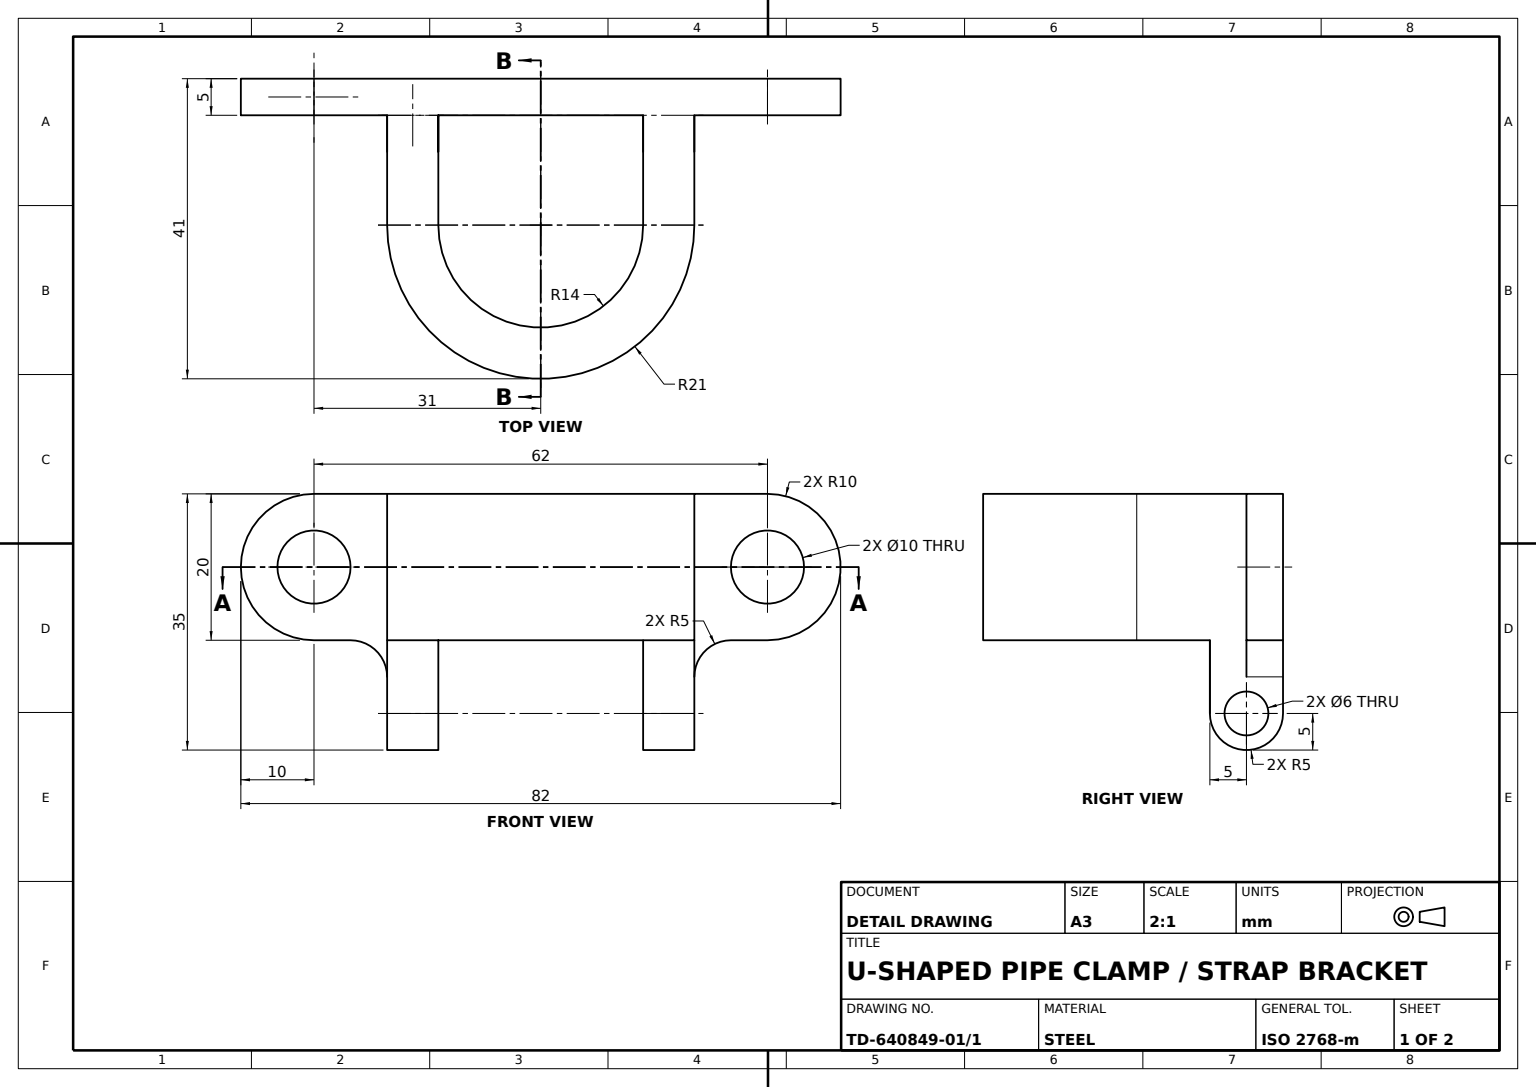
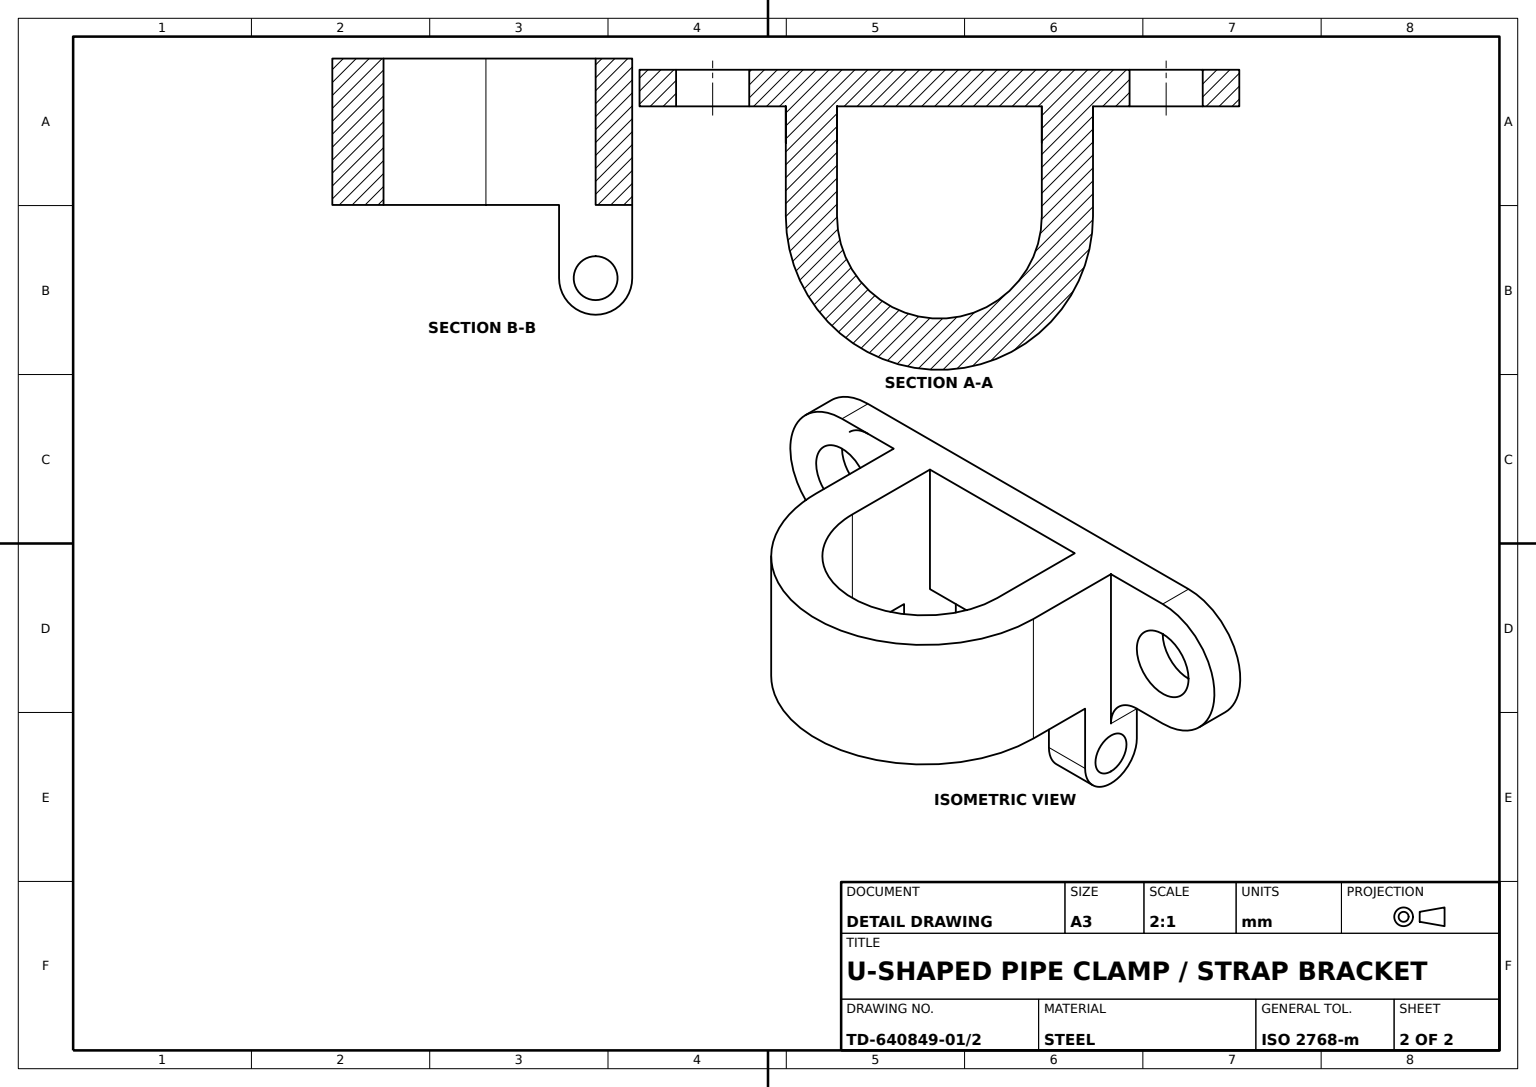
from build123d import *

# Parameters (mm, degrees)
BASE_FLANGE_DEPTH        = 5
CLAMP_BODY_DEPTH         = 20
BORE_28_DEPTH            = 20
FLANGE_CUT_SKETCH_R      = 5
FLANGE_CUT_DEPTH         = 20
LUG_A_DEPTH              = 5
LUG_A_WEB_SKETCH_W       = 5
LUG_A_WEB_SKETCH_H       = 10
LUG_A_WEB_DEPTH          = 7
LUG_B_DEPTH              = 5
LUG_BRIDGE_SKETCH_W      = 5
LUG_BRIDGE_SKETCH_H      = 10
LUG_BRIDGE_DEPTH         = 7
EAR_A_DEPTH              = 7
EAR_START                = -7
EAR_B_DEPTH              = 7
CLAMP_BOLT_HOLE_SKETCH_R = 3
CLAMP_BOLT_HOLE_6_DEPTH  = 70


with BuildPart() as part:
    # Base Flange Sketch → Base Flange (new body)
    with BuildSketch(Plane.XY):
        with BuildLine():
            Line((62, -10), (0, -10))
            ThreePointArc((0, -10), (-10, 0), (0, 10))
            Line((0, 10), (62, 10))
            ThreePointArc((62, 10), (72, 0), (62, -10))
        make_face()
    extrude(amount=BASE_FLANGE_DEPTH)

    # Clamp Body Sketch → Clamp Body (add)
    with BuildSketch(Plane.XZ.offset(10)):
        with BuildLine():
            Line((10, 5), (52, 5))
            Line((52, 5), (52, 20))
            ThreePointArc((52, 20), (31, 41), (10, 20))
            Line((10, 20), (10, 5))
        make_face()
    extrude(amount=-CLAMP_BODY_DEPTH)

    # Bore Sketch → Bore Ø28 (cut)
    with BuildSketch(Plane.XZ.offset(10)):
        with BuildLine():
            Line((17, 5), (17, 20))
            ThreePointArc((17, 20), (31, 34), (45, 20))
            Line((45, 20), (45, 5))
            Line((45, 5), (17, 5))
        make_face()
    extrude(amount=-BORE_28_DEPTH, mode=Mode.SUBTRACT)

    # Flange Cut Sketch → Flange Cut (cut)
    with BuildSketch(Plane.XY.offset(5)):
        with Locations((62, 0)):
            Circle(FLANGE_CUT_SKETCH_R)
        Circle(FLANGE_CUT_SKETCH_R)
    extrude(amount=-FLANGE_CUT_DEPTH, mode=Mode.SUBTRACT)

    # Lug A Sketch → Lug A (add)
    with BuildSketch(Plane.XY.offset(5)):
        with BuildLine():
            Line((10, -10), (5, -10))
            ThreePointArc((5, -10), (8.535533906, -11.464466094), (10, -15))
            Line((10, -15), (10, -20))
            Line((10, -20), (17, -20))
            Line((17, -20), (17, -10))
            Line((17, -10), (10, -10))
        make_face()
    extrude(amount=-LUG_A_DEPTH)

    # Lug A Web Sketch → Lug A Web (add)
    with BuildSketch(Plane(origin=(17, 0, 0), x_dir=(0, 0, -1), z_dir=(1, 0, 0))):
        with Locations((-7.5, -15)):
            Rectangle(LUG_A_WEB_SKETCH_W, LUG_A_WEB_SKETCH_H)
    extrude(amount=-LUG_A_WEB_DEPTH)

    # Lug B Sketch → Lug B (add)
    with BuildSketch(Plane.XY.offset(5)):
        with BuildLine():
            Line((52, -10), (57, -10))
            ThreePointArc((57, -10), (53.464466094, -11.464466094), (52, -15))
            Line((52, -15), (52, -20))
            Line((52, -20), (45, -20))
            Line((45, -20), (45, -10))
            Line((45, -10), (52, -10))
        make_face()
    extrude(amount=-LUG_B_DEPTH)

    # Lug Bridge Sketch → Lug Bridge (add)
    with BuildSketch(Plane.ZY.offset(-45)):
        with Locations((7.5, -15)):
            Rectangle(LUG_BRIDGE_SKETCH_W, LUG_BRIDGE_SKETCH_H)
    extrude(amount=-LUG_BRIDGE_DEPTH)

    # Ear A Sketch → Ear A (add)
    with BuildSketch(Plane.ZY.offset(-10)):
        with BuildLine():
            Line((0, -20), (10, -20))
            ThreePointArc((10, -20), (5, -25), (0, -20))
        make_face()
    extrude(amount=-EAR_A_DEPTH)

    # Ear B Sketch → Ear B (add)
    with BuildSketch(Plane(origin=(52, 0, 0), x_dir=(0, 0, -1), z_dir=(1, 0, 0)).offset(EAR_START)):
        with BuildLine():
            Line((-10, -20), (0, -20))
            ThreePointArc((0, -20), (-5, -25), (-10, -20))
        make_face()
    extrude(amount=EAR_B_DEPTH)

    # Clamp Bolt Hole Sketch → Clamp Bolt Hole Ø6 (cut)
    with BuildSketch(Plane(origin=(52, 0, 0), x_dir=(0, 0, -1), z_dir=(1, 0, 0))):
        with Locations(Location((-5, -20, 0), (0, 0, 90))):
            Circle(CLAMP_BOLT_HOLE_SKETCH_R)
    extrude(amount=-CLAMP_BOLT_HOLE_6_DEPTH, mode=Mode.SUBTRACT)


solid = part.part
